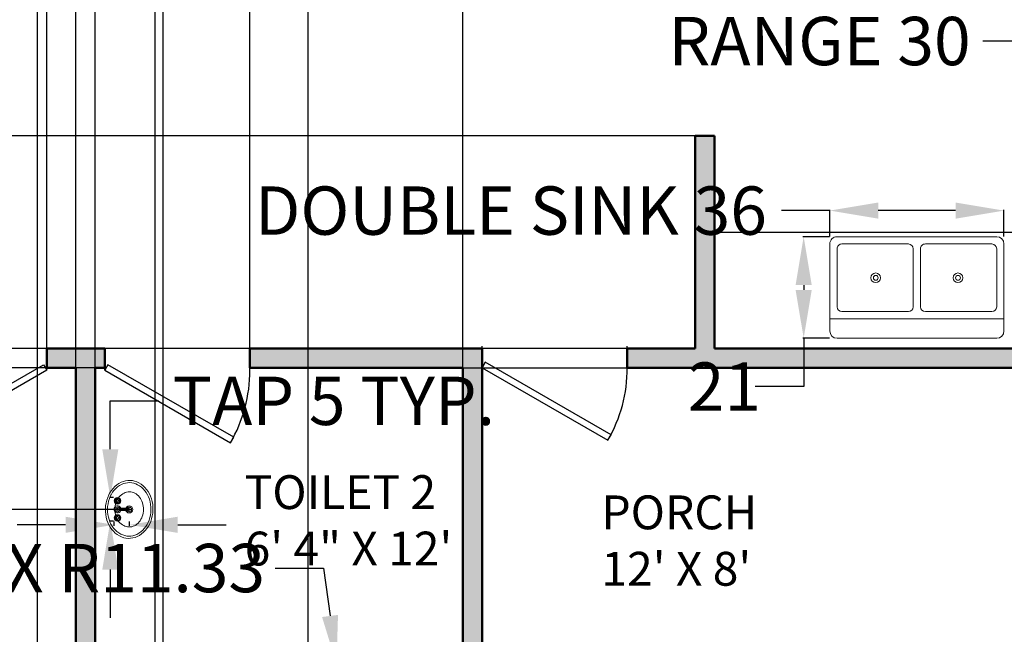
# Model space of a CAD drawing. Units: inches. Extents: x 133 to 758, y -29 to 543.
# Tile 3 of 7: x 386 to 590, y 108 to 235. Entities that reach past the tile are written whole.
import ezdxf

# ---------------------------------------------------------------- set-up
doc = ezdxf.new("R2010")
doc.units = ezdxf.units.IN
doc.header["$MEASUREMENT"] = 0
for name, color, linetype, lineweight in [('A-ANNO-DIMS', 2, 'Continuous', 18), ('A-AREA-IDEN', 7, 'Continuous', 25), ('A-FLOR-CASE', 32, 'Continuous', 25), ('A-FLOR-FIXT', 9, 'Continuous', 20), ('A-WALL', 7, 'Continuous', 50), ('DOOR', 40, 'Continuous', 25)]:
    doc.layers.add(name, color=color, linetype=linetype, lineweight=lineweight)
doc.layers.add('A-WALL-PATT', color=251, linetype='Continuous', lineweight=13, true_color=0x636466)
doc.styles.get("Standard").update_dxf_attribs({"font": 'arial.ttf'})
doc.dimstyles.get("Standard").update_dxf_attribs({"dimtxt": 10, "dimasz": 10, "dimexe": 0.18, "dimexo": 0.0625, "dimgap": 0.09, "dimtad": 0, "dimtih": 1, "dimtoh": 1, "dimdec": 0, "dimzin": 0, "dimdsep": 46, "dimlunit": 4, "dimtxsty": 'Standard', "dimcen": 0.09, "dimadec": 0, "dimazin": 0, "dimtfac": 1, "dimtdec": 0, "dimtofl": 0, "dimtmove": 0, "dimatfit": 3, "dimfxl": 1, "dimtolj": 1, "dimtzin": 0, "dimarcsym": 0})

# ---------------------------------------------------------------- blocks, each defined once
blk = doc.blocks.new('*U12')
for p, q in [((-40, 0), (-40, 6)), ((0, 0), (0, 6))]:
    blk.add_line(p, q)
blk.add_lwpolyline([(0, 0), (-34.64, -20), (-35.52, -18.48), (-0.88, 1.52)], close=True)
blk.add_arc((0, 0), 40, 180, 210)
blk = doc.blocks.new('*U13')
for p, q in [((0, 0), (0, 6)), ((40, 0), (40, 6))]:
    blk.add_line(p, q)
blk.add_lwpolyline([(0, 0), (34.64, -20), (35.52, -18.48), (0.87, 1.52)], close=True)
blk.add_arc((0, 0), 40, 330, 0)
blk = doc.blocks.new('Sink-double - 36 in top')
for p, q in [((-18, -4), (18, -4)), ((-0.75, -18.5), (-0.75, -6.5)), ((0.75, -6.5), (0.75, -18.5))]:
    blk.add_line(p, q)
for points in [[(-16.5, 0), (16.5, 0)], [(-18, -19.5), (-18, -1.5)], [(18, -1.5), (18, -19.5)], [(-15.5, -5.5), (-1.75, -5.5)], [(1.75, -5.5), (15.5, -5.5)], [(-16.5, -18.5), (-16.5, -6.5)], [(16.5, -6.5), (16.5, -18.5)], [(-1.75, -19.5), (-15.5, -19.5)], [(15.5, -19.5), (1.75, -19.5)], [(16.5, -21), (-16.5, -21)]]:
    blk.add_lwpolyline(points)
for centre, radius in [((-8.5, -12.5), 1), ((-8.5, -12.5), 0.5), ((8.5, -12.5), 1), ((8.5, -12.5), 0.5)]:
    blk.add_circle(centre, radius)
for centre, radius, start, end in [((-16.5, -1.5), 1.5, 90, 180), ((16.5, -1.5), 1.5, 0, 90), ((-15.5, -6.5), 1, 90, 180), ((-1.75, -6.5), 1, 0, 90), ((1.75, -6.5), 1, 90, 180), ((15.5, -6.5), 1, 0, 90), ((-16.5, -19.5), 1.5, 180, 270), ((-15.5, -18.5), 1, 180, 270), ((-1.75, -18.5), 1, 270, 0), ((1.75, -18.5), 1, 180, 270), ((15.5, -18.5), 1, 270, 0), ((16.5, -19.5), 1.5, 270, 0)]:
    blk.add_arc(centre, radius, start, end)
blk = doc.blocks.new('Sink - Oval top')
for p, q in [((-1, 0), (1, 0)), ((0, 1), (0, -1))]:
    blk.add_line(p, q)
for points in [[(-12.23, 0.39, 0.117634), (-11.46, -3.36, 0.104469), (-8.88, -6.8, 0.090016), (-5.08, -9.07, 0.08192), (-0.32, -10.02, 0.08192), (4.49, -9.38, 0.090016), (8.42, -7.36, 0.104469), (11.22, -4.09, 0.117634), (12.23, -0.39, 0.117634), (11.46, 3.36, 0.104469), (8.88, 6.8, 0.090016), (5.08, 9.07, 0.08192), (0.32, 10.02, 0.08192), (-4.49, 9.38, 0.090016), (-8.42, 7.36, 0.104469), (-11.22, 4.09, 0.117634)], [(-11.29, 0.16, 0.118622), (-10.52, -3.25, 0.104678), (-8.07, -6.36, 0.089562), (-4.54, -8.37, 0.081185), (-0.13, -9.15, 0.081185), (4.3, -8.49, 0.089562), (7.89, -6.58, 0.104678), (10.42, -3.55, 0.118622), (11.29, -0.16, 0.118622), (10.52, 3.25, 0.104678), (8.07, 6.36, 0.089562), (4.54, 8.37, 0.081185), (0.13, 9.15, 0.081185), (-4.3, 8.49, 0.089562), (-7.89, 6.58, 0.104678), (-10.42, 3.55, 0.118622)], [(-7.42, 0.08, 0.118283), (-6.91, -2.17, 0.104607), (-5.29, -4.21, 0.089718), (-2.97, -5.53, 0.081436), (-0.07, -6.04, 0.081436), (2.84, -5.59, 0.089718), (5.2, -4.33, 0.104607), (6.86, -2.32, 0.118283), (7.42, -0.08, 0.118283), (6.91, 2.17, 0.104607), (5.29, 4.21, 0.089718), (2.97, 5.53, 0.081436), (0.07, 6.04, 0.081436), (-2.84, 5.59, 0.089718), (-5.2, 4.33, 0.104607), (-6.86, 2.32, 0.118283)]]:
    blk.add_lwpolyline(points, format="xyb", close=True)
for radius in [1.5, 1]:
    blk.add_circle((0, 0), radius)
blk = doc.blocks.new('Faucet - Bathroom top')
for p, q in [((-4.107, 0.125), (-4.375, 0.125)), ((-3.75, 0.4788), (-3.75, 0.75)), ((-3.5, 0.482), (-3.5, 0.75)), ((-3.1461, 0.125), (-2.875, 0.125)), ((3.143, 0.125), (2.875, 0.125)), ((3.5, 0.4788), (3.5, 0.75)), ((3.75, 0.482), (3.75, 0.75)), ((4.1039, 0.125), (4.375, 0.125)), ((-4.1039, -0.125), (-4.375, -0.125)), ((-3.75, -0.4821), (-3.75, -0.75)), ((-3.5, -0.4789), (-3.5, -0.75)), ((-3.143, -0.125), (-2.875, -0.125)), ((-0.5, -0.8639), (-0.5, -4.5)), ((0.5, -4.5), (0.5, -0.8631)), ((3.1461, -0.125), (2.875, -0.125)), ((3.5, -0.4821), (3.5, -0.75)), ((3.75, -0.4789), (3.75, -0.75)), ((4.107, -0.125), (4.375, -0.125))]:
    blk.add_line(p, q)
for centre, radius in [((-3.625, 0), 1.375), ((-4.625, 0), 0.2795), ((-3.625, 0), 0.5), ((-3.625, 1), 0.2795), ((-2.625, 0), 0.2795), ((0, 0), 0.5), ((3.625, 0), 1.375), ((2.625, 0), 0.2795), ((3.625, 0), 0.5), ((3.625, 1), 0.2795), ((4.625, 0), 0.2795), ((-3.625, -1), 0.2795), ((3.625, -1), 0.2795)]:
    blk.add_circle(centre, radius)
for centre, radius, start, end in [((-3.625, 0), 1, 105.2407, 164.2093), ((-3.625, 0), 1, 16.44125, 74.07887), ((0, 0), 1.5, 289.6514, 250.3603), ((0, 0), 1, 300.3431, 239.7554), ((3.625, 0), 1, 106.12, 164.0884), ((3.625, 0), 1, 16.23422, 73.90469), ((-3.625, 0), 1, 196.2342, 253.9047), ((-3.625, 0), 1, 286.12, 344.0884), ((3.625, 0), 1, 196.4413, 254.0789), ((3.625, 0), 1, 285.2407, 344.2093), ((0, -4.5), 0.5, 180, 0)]:
    blk.add_arc(centre, radius, start, end)
blk = doc.blocks.new('*D54')
at = {"layer": 'A-ANNO-DIMS', "color": 0, "lineweight": -2, "transparency": 16777216}
for p, q in [((404.89, 146.5), (404.89, 156.5)), ((404.89, 156.5), (414.89, 156.5)), ((405.57, 136.5), (404.71, 136.5)), ((405.57, 131.6), (404.71, 131.6)), ((404.89, 121.6), (404.89, 111.6))]:
    blk.add_line(p, q, dxfattribs=at)
at = {"layer": 'A-ANNO-DIMS', "color": 0, "transparency": 16777216}
for points in [[(403.23, 146.5), (406.56, 146.5), (404.89, 136.5)], [(403.23, 121.6), (406.56, 121.6), (404.89, 131.6)]]:
    blk.add_solid(points, dxfattribs=at)
at = {"layer": 'Defpoints', "color": 0, "transparency": 16777216}
for p in [(404.89, 136.5), (405.63, 136.5), (405.63, 131.6)]:
    blk.add_point(p, dxfattribs=at)
at = {"layer": 'A-ANNO-DIMS', "color": 0, "transparency": 16777216, "insert": (451.09, 156.5), "char_height": 10, "attachment_point": 5}
blk.add_mtext('\\A1;TAP 5 TYP.', dxfattribs=at)
blk = doc.blocks.new('*D55')
at = {"layer": 'A-ANNO-DIMS', "color": 0, "lineweight": -2, "transparency": 16777216}
for p, q in [((395.63, 130.86), (385.63, 130.86)), ((405.63, 131.53), (405.63, 130.68)), ((408.82, 131.53), (408.82, 130.68)), ((418.82, 130.86), (428.82, 130.86))]:
    blk.add_line(p, q, dxfattribs=at)
at = {"layer": 'A-ANNO-DIMS', "color": 0, "transparency": 16777216}
for points in [[(395.63, 132.53), (395.63, 129.19), (405.63, 130.86)], [(418.82, 132.53), (418.82, 129.19), (408.82, 130.86)]]:
    blk.add_solid(points, dxfattribs=at)
at = {"layer": 'Defpoints', "color": 0, "transparency": 16777216}
for p in [(405.63, 131.6), (405.63, 130.86), (408.82, 131.6)]:
    blk.add_point(p, dxfattribs=at)
at = {"layer": 'A-ANNO-DIMS', "color": 0, "transparency": 16777216, "insert": (365.09, 130.86), "char_height": 10, "attachment_point": 5}
blk.add_mtext('\\A1;3 TYP.', dxfattribs=at)
blk = doc.blocks.new('*D62')
at = {"layer": 'A-ANNO-DIMS', "color": 0, "lineweight": -2, "transparency": 16777216}
for p, q in [((599.69, 270.92), (595.07, 270.92)), ((595.25, 260.92), (595.25, 250.92)), ((599.69, 240.92), (595.07, 240.92)), ((595.25, 240.92), (595.25, 230.92)), ((595.25, 230.92), (585.25, 230.92))]:
    blk.add_line(p, q, dxfattribs=at)
at = {"layer": 'A-ANNO-DIMS', "color": 0, "transparency": 16777216}
for points in [[(593.58, 260.92), (596.92, 260.92), (595.25, 270.92)], [(593.58, 250.92), (596.92, 250.92), (595.25, 240.92)]]:
    blk.add_solid(points, dxfattribs=at)
at = {"layer": 'Defpoints', "color": 0, "transparency": 16777216}
for p in [(599.75, 270.92), (595.25, 240.92), (599.75, 240.92)]:
    blk.add_point(p, dxfattribs=at)
at = {"layer": 'A-ANNO-DIMS', "color": 0, "transparency": 16777216, "insert": (551.49, 230.92), "char_height": 10, "attachment_point": 5}
blk.add_mtext('\\A1;RANGE 30', dxfattribs=at)
blk = doc.blocks.new('*D64')
at = {"layer": 'A-ANNO-DIMS', "color": 0, "lineweight": -2, "transparency": 16777216}
for p, q in [((553.61, 195.85), (543.61, 195.85)), ((553.61, 190.51), (553.61, 196.03)), ((579.61, 195.85), (563.61, 195.85)), ((589.61, 190.51), (589.61, 196.03))]:
    blk.add_line(p, q, dxfattribs=at)
at = {"layer": 'A-ANNO-DIMS', "color": 0, "transparency": 16777216}
for points in [[(563.61, 197.52), (563.61, 194.18), (553.61, 195.85)], [(579.61, 197.52), (579.61, 194.18), (589.61, 195.85)]]:
    blk.add_solid(points, dxfattribs=at)
at = {"layer": 'Defpoints', "color": 0, "transparency": 16777216}
for p in [(553.61, 195.85), (553.61, 190.45), (589.61, 190.45)]:
    blk.add_point(p, dxfattribs=at)
at = {"layer": 'A-ANNO-DIMS', "color": 0, "transparency": 16777216, "insert": (487.7, 195.85), "char_height": 10, "attachment_point": 5}
blk.add_mtext('\\A1;DOUBLE SINK 36', dxfattribs=at)
blk = doc.blocks.new('*D65')
at = {"layer": 'A-ANNO-DIMS', "color": 0, "lineweight": -2, "transparency": 16777216}
for p, q in [((553.54, 190.45), (548.03, 190.45)), ((548.21, 180.45), (548.21, 179.45)), ((553.54, 169.45), (548.03, 169.45)), ((548.21, 169.45), (548.21, 159.45)), ((548.21, 159.45), (538.21, 159.45))]:
    blk.add_line(p, q, dxfattribs=at)
at = {"layer": 'A-ANNO-DIMS', "color": 0, "transparency": 16777216}
for points in [[(546.54, 180.45), (549.87, 180.45), (548.21, 190.45)], [(546.54, 179.45), (549.87, 179.45), (548.21, 169.45)]]:
    blk.add_solid(points, dxfattribs=at)
at = {"layer": 'Defpoints', "color": 0, "transparency": 16777216}
for p in [(553.61, 190.45), (548.21, 169.45), (553.61, 169.45)]:
    blk.add_point(p, dxfattribs=at)
at = {"layer": 'A-ANNO-DIMS', "color": 0, "transparency": 16777216, "insert": (531.83, 159.45), "char_height": 10, "attachment_point": 5}
blk.add_mtext('\\A1;21', dxfattribs=at)
blk = doc.blocks.new('*D75')
at = {"layer": 'A-ANNO-DIMS', "color": 0, "lineweight": -2, "transparency": 16777216}
for p, q in [((525.69, 307.34), (231.17, 307.34)), ((231.35, 297.34), (231.35, 264.53)), ((231.35, 221.34), (231.35, 254.14)), ((525.69, 211.34), (231.17, 211.34))]:
    blk.add_line(p, q, dxfattribs=at)
at = {"layer": 'A-ANNO-DIMS', "color": 0, "transparency": 16777216}
for points in [[(229.68, 297.34), (233.02, 297.34), (231.35, 307.34)], [(229.68, 221.34), (233.02, 221.34), (231.35, 211.34)]]:
    blk.add_solid(points, dxfattribs=at)
at = {"layer": 'Defpoints', "color": 0, "transparency": 16777216}
for p in [(231.35, 307.34), (525.75, 307.34), (525.75, 211.34)]:
    blk.add_point(p, dxfattribs=at)
at = {"layer": 'A-ANNO-DIMS', "color": 0, "transparency": 16777216, "insert": (231.35, 259.34), "char_height": 10, "attachment_point": 5}
blk.add_mtext('\\A1;96', dxfattribs=at)
blk = doc.blocks.new('*D76')
at = {"layer": 'A-ANNO-DIMS', "color": 0, "lineweight": -2, "transparency": 16777216}
for p, q in [((525.69, 211.34), (231.17, 211.34)), ((231.35, 201.34), (231.35, 194.43)), ((231.35, 177.34), (231.35, 184.25)), ((525.69, 167.34), (231.17, 167.34))]:
    blk.add_line(p, q, dxfattribs=at)
at = {"layer": 'A-ANNO-DIMS', "color": 0, "transparency": 16777216}
for points in [[(229.68, 201.34), (233.02, 201.34), (231.35, 211.34)], [(229.68, 177.34), (233.02, 177.34), (231.35, 167.34)]]:
    blk.add_solid(points, dxfattribs=at)
at = {"layer": 'Defpoints', "color": 0, "transparency": 16777216}
for p in [(231.35, 211.34), (525.75, 211.34), (525.75, 167.34)]:
    blk.add_point(p, dxfattribs=at)
at = {"layer": 'A-ANNO-DIMS', "color": 0, "transparency": 16777216, "insert": (231.35, 189.34), "char_height": 10, "attachment_point": 5}
blk.add_mtext('\\A1;44', dxfattribs=at)
blk = doc.blocks.new('*D78')
at = {"layer": 'A-ANNO-DIMS', "color": 0, "lineweight": -2, "transparency": 16777216}
for p, q in [((361.75, 167.4), (361.75, 533.92)), ((371.75, 533.74), (381.75, 533.74)), ((391.75, 167.4), (391.75, 533.92)), ((391.75, 533.74), (401.75, 533.74))]:
    blk.add_line(p, q, dxfattribs=at)
at = {"layer": 'A-ANNO-DIMS', "color": 0, "transparency": 16777216}
for points in [[(371.75, 535.4), (371.75, 532.07), (361.75, 533.74)], [(381.75, 535.4), (381.75, 532.07), (391.75, 533.74)]]:
    blk.add_solid(points, dxfattribs=at)
at = {"layer": 'Defpoints', "color": 0, "transparency": 16777216}
for p in [(391.75, 533.74), (361.75, 167.34), (391.75, 167.34)]:
    blk.add_point(p, dxfattribs=at)
at = {"layer": 'A-ANNO-DIMS', "color": 0, "transparency": 16777216, "insert": (408.98, 533.74), "char_height": 10, "attachment_point": 5}
blk.add_mtext('\\A1;30', dxfattribs=at)
blk = doc.blocks.new('*D85')
at = {"layer": 'A-ANNO-DIMS', "color": 0, "lineweight": -2, "transparency": 16777216}
for p, q in [((389.75, 399.27), (389.75, -22.24)), ((415.75, 399.27), (415.75, -22.24)), ((389.75, -22.06), (379.75, -22.06)), ((405.75, -22.06), (399.75, -22.06))]:
    blk.add_line(p, q, dxfattribs=at)
at = {"layer": 'A-ANNO-DIMS', "color": 0, "transparency": 16777216}
for points in [[(399.75, -20.4), (399.75, -23.73), (389.75, -22.06)], [(405.75, -20.4), (405.75, -23.73), (415.75, -22.06)]]:
    blk.add_solid(points, dxfattribs=at)
at = {"layer": 'Defpoints', "color": 0, "transparency": 16777216}
for p in [(389.75, 399.34), (415.75, 399.34), (389.75, -22.06)]:
    blk.add_point(p, dxfattribs=at)
at = {"layer": 'A-ANNO-DIMS', "color": 0, "transparency": 16777216, "insert": (372.42, -22.06), "char_height": 10, "attachment_point": 5}
blk.add_mtext('\\A1;26', dxfattribs=at)
blk = doc.blocks.new('*D89')
at = {"layer": 'A-ANNO-DIMS', "color": 0, "lineweight": -2, "transparency": 16777216}
for p, q in [((387.75, 533.74), (377.75, 533.74)), ((397.75, 163.4), (397.75, 533.92)), ((401.75, 163.4), (401.75, 533.92)), ((411.75, 533.74), (421.75, 533.74))]:
    blk.add_line(p, q, dxfattribs=at)
at = {"layer": 'A-ANNO-DIMS', "color": 0, "transparency": 16777216}
for points in [[(387.75, 535.4), (387.75, 532.07), (397.75, 533.74)], [(411.75, 535.4), (411.75, 532.07), (401.75, 533.74)]]:
    blk.add_solid(points, dxfattribs=at)
at = {"layer": 'Defpoints', "color": 0, "transparency": 16777216}
for p in [(401.75, 533.74), (397.75, 163.34), (401.75, 163.34)]:
    blk.add_point(p, dxfattribs=at)
at = {"layer": 'A-ANNO-DIMS', "color": 0, "transparency": 16777216, "insert": (425.3, 533.74), "char_height": 10, "attachment_point": 5}
blk.add_mtext('\\A1;4', dxfattribs=at)
blk = doc.blocks.new('*D90')
at = {"layer": 'A-ANNO-DIMS', "color": 0, "lineweight": -2, "transparency": 16777216}
for p, q in [((433.75, 167.4), (433.75, 533.92)), ((443.75, 533.74), (448.32, 533.74)), ((467.75, 533.74), (463.18, 533.74)), ((477.75, 163.4), (477.75, 533.92))]:
    blk.add_line(p, q, dxfattribs=at)
at = {"layer": 'A-ANNO-DIMS', "color": 0, "transparency": 16777216}
for points in [[(443.75, 535.4), (443.75, 532.07), (433.75, 533.74)], [(467.75, 535.4), (467.75, 532.07), (477.75, 533.74)]]:
    blk.add_solid(points, dxfattribs=at)
at = {"layer": 'Defpoints', "color": 0, "transparency": 16777216}
for p in [(477.75, 533.74), (433.75, 167.34), (477.75, 163.34)]:
    blk.add_point(p, dxfattribs=at)
at = {"layer": 'A-ANNO-DIMS', "color": 0, "transparency": 16777216, "insert": (455.75, 533.74), "char_height": 10, "attachment_point": 5}
blk.add_mtext('\\A1;44', dxfattribs=at)
blk = doc.blocks.new('*D91')
at = {"layer": 'A-ANNO-DIMS', "color": 0, "lineweight": -2, "transparency": 16777216}
for p, q in [((415.75, 399.27), (415.75, -22.24)), ((445.75, 399.27), (445.75, -22.24)), ((425.75, -22.06), (435.75, -22.06)), ((445.75, -22.06), (455.75, -22.06))]:
    blk.add_line(p, q, dxfattribs=at)
at = {"layer": 'A-ANNO-DIMS', "color": 0, "transparency": 16777216}
for points in [[(425.75, -20.4), (425.75, -23.73), (415.75, -22.06)], [(435.75, -20.4), (435.75, -23.73), (445.75, -22.06)]]:
    blk.add_solid(points, dxfattribs=at)
at = {"layer": 'Defpoints', "color": 0, "transparency": 16777216}
for p in [(415.75, 399.34), (445.75, 399.34), (445.75, -22.06)]:
    blk.add_point(p, dxfattribs=at)
at = {"layer": 'A-ANNO-DIMS', "color": 0, "transparency": 16777216, "insert": (462.98, -22.06), "char_height": 10, "attachment_point": 5}
blk.add_mtext('\\A1;30', dxfattribs=at)
blk = doc.blocks.new('*D93')
at = {"layer": 'A-ANNO-DIMS', "color": 0, "lineweight": -2, "transparency": 16777216}
for p, q in [((477.81, 163.34), (660.33, 163.34)), ((660.15, 153.34), (660.15, 139.65)), ((660.15, 115.57), (660.15, 129.26)), ((475.03, 105.57), (660.33, 105.57))]:
    blk.add_line(p, q, dxfattribs=at)
at = {"layer": 'A-ANNO-DIMS', "color": 0, "transparency": 16777216}
for points in [[(658.48, 153.34), (661.82, 153.34), (660.15, 163.34)], [(658.48, 115.57), (661.82, 115.57), (660.15, 105.57)]]:
    blk.add_solid(points, dxfattribs=at)
at = {"layer": 'Defpoints', "color": 0, "transparency": 16777216}
for p in [(477.75, 163.34), (660.15, 163.34), (474.97, 105.57)]:
    blk.add_point(p, dxfattribs=at)
at = {"layer": 'A-ANNO-DIMS', "color": 0, "transparency": 16777216, "insert": (660.15, 134.45), "char_height": 10, "attachment_point": 5}
blk.add_mtext('\\A1;57.76', dxfattribs=at)
blk = doc.blocks.new('*D96')
at = {"layer": 'A-ANNO-DIMS', "color": 0, "lineweight": -2, "transparency": 16777216}
for p, q in [((231.35, 163.34), (231.35, 173.34)), ((231.35, 173.34), (241.35, 173.34)), ((401.69, 163.34), (231.17, 163.34)), ((231.35, 144.05), (231.35, 153.34)), ((408.73, 134.05), (231.17, 134.05))]:
    blk.add_line(p, q, dxfattribs=at)
at = {"layer": 'A-ANNO-DIMS', "color": 0, "transparency": 16777216}
for points in [[(229.68, 153.34), (233.02, 153.34), (231.35, 163.34)], [(229.68, 144.05), (233.02, 144.05), (231.35, 134.05)]]:
    blk.add_solid(points, dxfattribs=at)
at = {"layer": 'Defpoints', "color": 0, "transparency": 16777216}
for p in [(231.35, 163.34), (401.75, 163.34), (408.8, 134.05)]:
    blk.add_point(p, dxfattribs=at)
at = {"layer": 'A-ANNO-DIMS', "color": 0, "transparency": 16777216, "insert": (258.41, 173.34), "char_height": 10, "attachment_point": 5}
blk.add_mtext('\\A1;29.29', dxfattribs=at)
blk = doc.blocks.new('*D99')
at = {"layer": 'A-ANNO-DIMS', "color": 0, "lineweight": -2, "transparency": 16777216}
for p, q in [((391.75, 533.74), (381.75, 533.74)), ((401.75, 19.4), (401.75, 533.92)), ((414.17, 21.95), (414.17, 533.92)), ((424.17, 533.74), (434.17, 533.74))]:
    blk.add_line(p, q, dxfattribs=at)
at = {"layer": 'A-ANNO-DIMS', "color": 0, "transparency": 16777216}
for points in [[(391.75, 535.4), (391.75, 532.07), (401.75, 533.74)], [(424.17, 535.4), (424.17, 532.07), (414.17, 533.74)]]:
    blk.add_solid(points, dxfattribs=at)
at = {"layer": 'Defpoints', "color": 0, "transparency": 16777216}
for p in [(401.75, 533.74), (414.17, 21.89), (401.75, 19.34)]:
    blk.add_point(p, dxfattribs=at)
at = {"layer": 'A-ANNO-DIMS', "color": 0, "transparency": 16777216, "insert": (361.37, 533.74), "char_height": 10, "attachment_point": 5}
blk.add_mtext('\\A1;12.417', dxfattribs=at)
blk = doc.blocks.new('*D102')
at = {"layer": 'A-ANNO-DIMS', "color": 0, "lineweight": -2, "transparency": 16777216}
for p, q in [((438.98, 121.92), (448.98, 121.92)), ((448.98, 121.92), (450.31, 112.01)), ((453.06, 90.87), (453.24, 90.87)), ((453.15, 90.78), (453.15, 90.96))]:
    blk.add_line(p, q, dxfattribs=at)
at = {"layer": 'A-ANNO-DIMS', "color": 0, "transparency": 16777216}
blk.add_solid([(451.96, 112.23), (448.66, 111.79), (451.64, 102.1)], dxfattribs=at)
at = {"layer": 'Defpoints', "color": 0, "transparency": 16777216}
for p in [(451.64, 102.1), (453.15, 90.87)]:
    blk.add_point(p, dxfattribs=at)
at = {"layer": 'A-ANNO-DIMS', "color": 0, "transparency": 16777216, "insert": (406.29, 121.92), "char_height": 10, "attachment_point": 5}
blk.add_mtext('\\A1;4X R11.33', dxfattribs=at)

msp = doc.modelspace()

# ---------------------------------------------------------------- hatches: boundary and pattern name
at = {"layer": 'A-WALL-PATT'}
h = msp.add_hatch(color=256, dxfattribs=at)
h.dxf.hatch_style = 1
h.paths.add_polyline_path([(634.7501, 235.336), (625.7501, 235.336), (625.7501, 167.336), (529.7501, 167.336), (529.7501, 211.336), (525.7501, 211.336), (525.7501, 167.336), (511.7501, 167.336), (511.7501, 163.336), (625.7501, 163.336), (625.7501, 19.336), (625.1804, 19.336), (601.3503, 19.336), (601.3503, 17.336), (601.3503, 10.336), (634.7501, 10.336)])
h = msp.add_hatch(color=256, dxfattribs=at)
h.dxf.hatch_style = 1
h.paths.add_polyline_path([(425.9734, 19.336), (401.7501, 19.336), (401.7501, 163.336), (403.7501, 163.336), (403.7501, 167.336), (391.7501, 167.336), (391.7501, 163.336), (397.7501, 163.336), (397.7501, 19.336), (357.4362, 19.336), (357.4362, 10.336), (425.9734, 10.336)])
h = msp.add_hatch(color=256, dxfattribs=at)
h.dxf.hatch_style = 1
h.paths.add_polyline_path([(505.7501, 17.336), (505.7501, 19.336), (481.7501, 19.336), (481.7501, 67.336), (481.7501, 163.336), (481.7501, 167.336), (433.7501, 167.336), (433.7501, 163.336), (477.7501, 163.336), (477.7501, 19.336), (449.9734, 19.336), (449.9734, 10.336), (505.7501, 10.336)])

# ---------------------------------------------------------------- linework, layer by layer
at = {"layer": 'A-FLOR-CASE'}
msp.add_line((601.7501, 191.336), (529.7501, 191.336), dxfattribs=at)
at = {"layer": 'A-WALL'}
for p, q in [((529.7501, 211.336), (525.7501, 211.336)), ((525.7501, 211.336), (525.7501, 167.336)), ((529.7501, 211.336), (529.7501, 167.336)), ((391.7501, 163.336), (391.7501, 167.336)), ((403.7501, 167.336), (391.7501, 167.336)), ((403.7501, 163.336), (403.7501, 167.336)), ((481.7501, 167.336), (433.7501, 167.336)), ((433.7501, 163.336), (433.7501, 167.336)), ((481.7501, 163.336), (481.7501, 167.336)), ((525.7501, 167.336), (511.7501, 167.336)), ((511.7501, 163.336), (511.7501, 167.336)), ((625.7501, 167.336), (529.7501, 167.336)), ((397.7501, 163.336), (391.7501, 163.336)), ((397.7501, 19.336), (397.7501, 163.336)), ((401.7501, 19.336), (401.7501, 163.336)), ((403.7501, 163.336), (401.7501, 163.336)), ((477.7501, 163.336), (433.7501, 163.336)), ((477.7501, 19.336), (477.7501, 163.336)), ((481.7501, 19.336), (481.7501, 163.336)), ((625.7501, 163.336), (511.7501, 163.336))]:
    msp.add_line(p, q, dxfattribs=at)

# ---------------------------------------------------------------- block references
at = {"layer": 'A-FLOR-FIXT', "rotation": 180}
msp.add_blockref('Sink-double - 36 in top', (571.6062, 169.4488), dxfattribs=at)
at = {"layer": 'A-FLOR-FIXT', "xscale": 0.4902491559291568, "yscale": 0.4902491559291568, "zscale": 0.4902491559291568, "rotation": 90}
for name, p in [('Sink - Oval top', (408.7964, 134.0481)), ('Faucet - Bathroom top', (406.3653, 134.0477))]:
    msp.add_blockref(name, p, dxfattribs=at)
at = {"layer": 'DOOR', "xscale": 0.75, "yscale": 0.75, "zscale": 0.75}
for name, p in [('*U12', (391.7501, 162.836)), ('*U13', (403.7501, 162.836)), ('*U13', (481.7501, 163.336))]:
    msp.add_blockref(name, p, dxfattribs=at)

# ---------------------------------------------------------------- texts
at = {"layer": 'A-AREA-IDEN', "char_height": 7, "attachment_point": 1}
for s, width, insert in [('TOILET 2\\P6\' 4" X 12\'', 69.65376, (432.6571, 141.1156)), ("PORCH\\P12' X 8'", 109.060718, (506.4032, 136.9361))]:
    msp.add_mtext_dynamic_manual_height_columns(s, width=width, gutter_width=1, heights=[0], dxfattribs=dict(at, insert=insert))

# ---------------------------------------------------------------- dimensions: what is measured, and where the dimension line sits
at = {"layer": 'A-ANNO-DIMS'}
for base, p1, p2, override, picture, middle in [((401.75012, 533.73604), (414.16755, 21.88596), (401.75012, 19.33604), {"dimdec": 3, "dimlfac": 1, "dimrnd": 0, "dimzin": 0, "dimdsep": 46, "dimlunit": 2}, '*D99', (361.37362, 533.73604)), ((391.7501, 533.736), (361.7501, 167.336), (391.7501, 167.336), {"dimdec": 0, "dimlfac": 1, "dimrnd": 0, "dimzin": 0, "dimdsep": 46, "dimlunit": 2}, '*D78', (408.982, 533.736)), ((401.7501, 533.736), (397.7501, 163.336), (401.7501, 163.336), {"dimdec": 0, "dimlfac": 1, "dimrnd": 0, "dimzin": 0, "dimdsep": 46, "dimlunit": 2}, '*D89', (425.2985, 533.736)), ((477.7501, 533.736), (433.7501, 167.336), (477.7501, 163.336), {"dimdec": 0, "dimlfac": 1, "dimrnd": 0, "dimzin": 0, "dimdsep": 46, "dimlunit": 2}, '*D90', (455.7501, 533.736)), ((389.7501, -22.064), (415.7501, 399.336), (389.7501, 399.336), {"dimdec": 0, "dimlfac": 1, "dimrnd": 0, "dimzin": 0, "dimdsep": 46, "dimlunit": 2}, '*D85', (372.4159, -22.064)), ((445.7501, -22.064), (415.7501, 399.336), (445.7501, 399.336), {"dimdec": 0, "dimlfac": 1, "dimrnd": 0, "dimzin": 0, "dimdsep": 46, "dimlunit": 2}, '*D91', (462.982, -22.064))]:
    dim = msp.add_linear_dim(base=base, p1=p1, p2=p2, dimstyle='Standard', override=override, dxfattribs=at)
    dim.commit()
    dim.dimension.update_dxf_attribs({"geometry": picture, "text_midpoint": middle})
for base, p1, p2, angle, override, picture, middle in [((231.3501, 307.336), (525.7501, 211.336), (525.7501, 307.336), 90, {"dimdec": 0, "dimlfac": 1, "dimrnd": 0, "dimzin": 0, "dimdsep": 46, "dimlunit": 2}, '*D75', (231.3501, 259.336)), ((231.3501, 211.336), (525.7501, 167.336), (525.7501, 211.336), 90, {"dimdec": 0, "dimlfac": 1, "dimrnd": 0, "dimzin": 0, "dimdsep": 46, "dimlunit": 2}, '*D76', (231.3501, 189.336)), ((548.2062, 169.4488), (553.6062, 190.4488), (553.6062, 169.4488), 270, {"dimdec": 0, "dimlfac": 1, "dimrnd": 0, "dimzin": 0, "dimdsep": 46, "dimlunit": 2}, '*D65', (531.8338, 159.4488)), ((231.3501, 163.336), (408.7964, 134.0481), (401.7501, 163.336), 90, {"dimdec": 2, "dimlfac": 1, "dimrnd": 0, "dimzin": 0, "dimdsep": 46, "dimlunit": 2}, '*D96', (258.4081, 173.336)), ((660.1501, 163.336), (474.9703, 105.5711), (477.7501, 163.336), 90, {"dimdec": 2, "dimlfac": 1, "dimrnd": 0, "dimzin": 0, "dimdsep": 46, "dimlunit": 2}, '*D93', (660.1501, 134.4536))]:
    dim = msp.add_linear_dim(base=base, p1=p1, p2=p2, angle=angle, dimstyle='Standard', override=override, dxfattribs=at)
    dim.commit()
    dim.dimension.update_dxf_attribs({"geometry": picture, "text_midpoint": middle})
for base, p1, p2, angle, text, picture, middle in [((595.2501, 240.9203), (599.7501, 270.9203), (599.7501, 240.9203), 270, 'RANGE <>', '*D62', (551.4937, 230.9203)), ((553.6062, 195.8488), (589.6062, 190.4488), (553.6062, 190.4488), 180, 'DOUBLE SINK <>', '*D64', (487.6976, 195.8488)), ((404.8945, 136.499), (405.6299, 131.5965), (405.6299, 136.499), 90, 'TAP <> TYP.', '*D54', (451.0895, 156.499)), ((405.6299, 130.8611), (408.8165, 131.5965), (405.6299, 131.5965), 180, '<> TYP.', '*D55', (365.0897, 130.8611))]:
    dim = msp.add_linear_dim(base=base, p1=p1, p2=p2, angle=angle, text=text, dimstyle='Standard', override={"dimdec": 0, "dimlfac": 1, "dimrnd": 0, "dimzin": 0, "dimdsep": 46, "dimlunit": 2}, dxfattribs=at)
    dim.commit()
    dim.dimension.update_dxf_attribs({"geometry": picture, "text_midpoint": middle})
dim = msp.add_radius_dim(center=(453.1529, 90.8712), mpoint=(451.643, 102.0993), text='4X <>', dimstyle='Standard', override={"dimdec": 2, "dimlfac": 1, "dimrnd": 0, "dimzin": 0, "dimdsep": 46, "dimlunit": 2}, dxfattribs=at)
dim.commit()
dim.dimension.update_dxf_attribs({"geometry": '*D102', "text_midpoint": (406.2851, 121.9209)})

doc.saveas('drawing.dxf')
